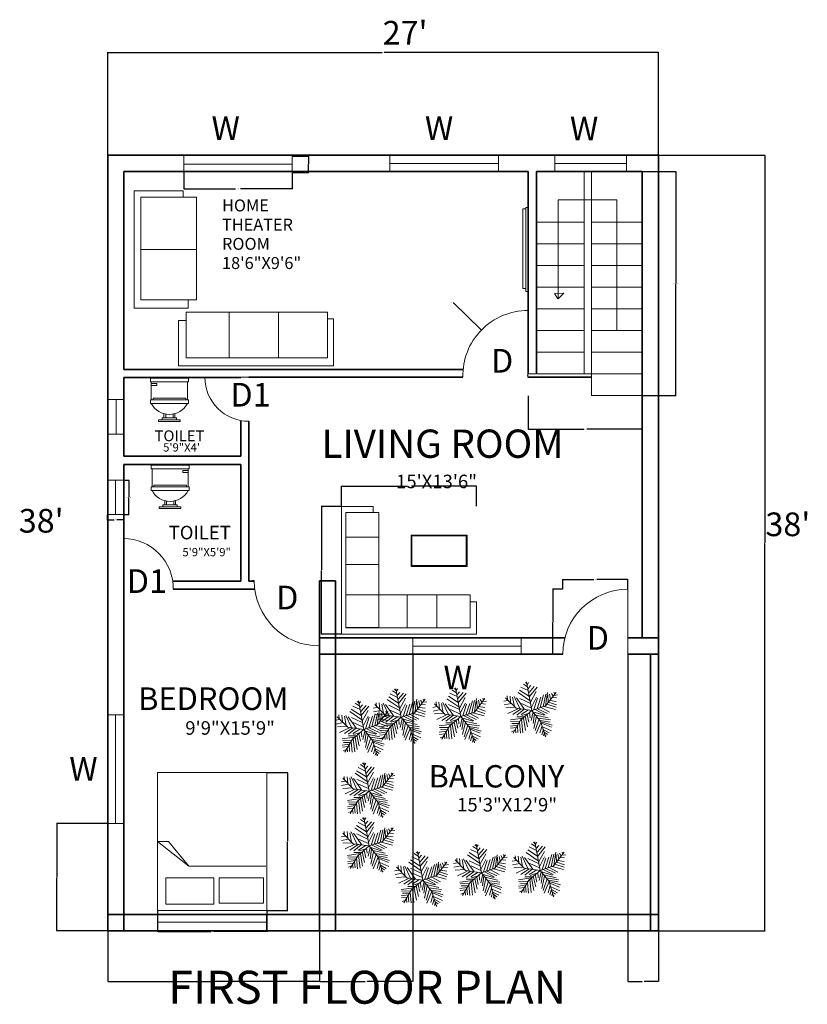
# Model space of a CAD drawing. Units: inches. Extents: x -26 to 788, y -42 to 505.
# Tile 9 of 9: x 353 to 788, y -40 to 505. Entities that reach past the tile are written whole.
import ezdxf

# ---------------------------------------------------------------- set-up
doc = ezdxf.new("R2010")
doc.units = ezdxf.units.IN
doc.header["$MEASUREMENT"] = 0
for name, color, linetype, lineweight in [('A-ANNO-DIMS', 2, 'Continuous', 18), ('A-ANNO-IDEN', 3, 'Continuous', 18), ('A-ANNO-TEXT', 7, 'Continuous', 25), ('A-AREA-IDEN', 7, 'Continuous', 18), ('A-DOOR', 3, 'Continuous', 18), ('A-EQPM', 8, 'Continuous', 18), ('A-FLOR-FIXT', 9, 'Continuous', 18), ('A-FLOR-STRS', 7, 'Continuous', 18), ('A-FURN', 8, 'Continuous', 18), ('A-GLAZ', 4, 'Continuous', 18), ('A-WALL', 7, 'Continuous', 35), ('L-PLNT', 94, 'Continuous', 13)]:
    doc.layers.add(name, color=color, linetype=linetype, lineweight=lineweight)
doc.styles.get("Standard").update_dxf_attribs({"font": 'arial.ttf'})
doc.dimstyles.get("Standard").update_dxf_attribs({"dimtxt": 0.18, "dimasz": 0.18, "dimexe": 0.18, "dimexo": 0.0625, "dimgap": 0.09, "dimtad": 0, "dimtih": 1, "dimtoh": 1, "dimdec": 4, "dimzin": 0, "dimdsep": 46, "dimtxsty": 'Standard', "dimcen": 0.09, "dimadec": 0, "dimazin": 0, "dimtfac": 1, "dimtdec": 4, "dimtofl": 0, "dimtmove": 0, "dimatfit": 3, "dimfxl": 1, "dimtolj": 1, "dimtzin": 0, "dimarcsym": 0})

# ---------------------------------------------------------------- blocks, each defined once
blk = doc.blocks.new('*U2')
for p, q in [((-10, 22), (-10, 12)), ((10, 12), (10, 22)), ((-10, 21), (-7, 21)), ((-7, 20), (-10, 20)), ((-7, 21), (-7, 20)), ((10.5, 12), (-10.5, 12)), ((-10.5, 10), (-10.5, 12)), ((9, 13), (-9, 13)), ((-9, 13), (-9, 12)), ((9, 12), (9, 13)), ((10.5, 12), (10.5, 10)), ((10.5, 10), (-10.5, 10)), ((4, 2), (-4, 2)), ((-4, 2), (-4, 1)), ((-3, 4.4065), (-3, 2)), ((-2, 2), (-2, 4.1658)), ((2, 4.1658), (2, 2)), ((3, 2), (3, 4.4065)), ((4, 1), (4, 2))]:
    blk.add_line(p, q)
for points in [[(10.5, 22), (10.5, 24), (-10.5, 24), (-10.5, 22)], [(6, 0), (6, 1), (-6, 1), (-6, 0)]]:
    blk.add_lwpolyline(points, close=True)
blk.add_arc((0, 15.3333), 11.3333, 208.0725, 331.9275)
blk = doc.blocks.new('*U3')
for p, q in [((-10, 12), (-10, 22)), ((10, 22), (10, 12)), ((10, 21), (7, 21)), ((7, 21), (7, 20)), ((7, 20), (10, 20)), ((-10.5, 12), (10.5, 12)), ((-10.5, 12), (-10.5, 10)), ((-9, 13), (9, 13)), ((-9, 12), (-9, 13)), ((9, 13), (9, 12)), ((10.5, 10), (10.5, 12)), ((-10.5, 10), (10.5, 10)), ((-4, 2), (4, 2)), ((-4, 1), (-4, 2)), ((-3, 2), (-3, 4.4065)), ((-2, 4.1658), (-2, 2)), ((2, 2), (2, 4.1658)), ((3, 4.4065), (3, 2)), ((4, 2), (4, 1))]:
    blk.add_line(p, q)
for points in [[(-10.5, 22), (-10.5, 24), (10.5, 24), (10.5, 22)], [(-6, 0), (-6, 1), (6, 1), (6, 0)]]:
    blk.add_lwpolyline(points, close=True)
blk.add_arc((0, 15.3333), 11.3333, 208.0725, 331.9275)
blk = doc.blocks.new('*D5')
at = {"layer": 'A-ANNO-DIMS', "color": 0, "lineweight": -2, "transparency": 16777216}
for p, q in [((401.21, 429.6), (401.21, 486.57)), ((401.39, 486.39), (552.86, 486.39)), ((705.53, 486.39), (554.07, 486.39)), ((705.71, 429.6), (705.71, 486.57))]:
    blk.add_line(p, q, dxfattribs=at)
at = {"layer": 'A-ANNO-DIMS', "color": 0, "transparency": 16777216}
for points in [[(401.39, 486.42), (401.39, 486.36), (401.21, 486.39)], [(705.53, 486.42), (705.53, 486.36), (705.71, 486.39)]]:
    blk.add_solid(points, dxfattribs=at)
at = {"layer": 'Defpoints', "color": 0, "transparency": 16777216}
for p in [(705.71, 486.39), (401.21, 429.53), (705.71, 429.53)]:
    blk.add_point(p, dxfattribs=at)
at = {"layer": 'A-ANNO-DIMS', "color": 0, "transparency": 16777216, "insert": (553.46, 486.39), "char_height": 0.18, "attachment_point": 5}
blk.add_mtext('\\A1;304.5000', dxfattribs=at)
blk = doc.blocks.new('*D6')
at = {"layer": 'A-ANNO-DIMS', "color": 0, "lineweight": -2, "transparency": 16777216}
for p, q in [((705.78, 429.53), (764.6, 429.53)), ((764.42, 429.35), (764.42, 215.21)), ((764.42, 0.71), (764.42, 214.85)), ((705.78, 0.53), (764.6, 0.53))]:
    blk.add_line(p, q, dxfattribs=at)
at = {"layer": 'A-ANNO-DIMS', "color": 0, "transparency": 16777216}
for points in [[(764.39, 429.35), (764.45, 429.35), (764.42, 429.53)], [(764.39, 0.71), (764.45, 0.71), (764.42, 0.53)]]:
    blk.add_solid(points, dxfattribs=at)
at = {"layer": 'Defpoints', "color": 0, "transparency": 16777216}
for p in [(705.71, 429.53), (705.71, 0.53), (764.42, 0.53)]:
    blk.add_point(p, dxfattribs=at)
at = {"layer": 'A-ANNO-DIMS', "color": 0, "transparency": 16777216, "insert": (764.42, 215.03), "char_height": 0.18, "attachment_point": 5}
blk.add_mtext('\\A1;429.0000', dxfattribs=at)
blk = doc.blocks.new('*U11')
for p, q in [((-129.8956, 713.6638), (-626.7704, 1032.1544)), ((-185.1152, 1008.5578), (-553.1612, 1185.4942)), ((-221.9198, 1197.3052), (-433.5526, 1338.8594)), ((-258.7244, 1362.456), (-332.3336, 1421.4348)), ((0, 0), (-266.7, 1447.8)), ((-231.1146, 1315.2628), (-166.7002, 1421.4348)), ((-194.31, 1102.9442), (-65.4812, 1256.284)), ((-148.3106, 914.1968), (118.5418, 1220.9018)), ((-129.8956, 701.8528), (265.7602, 1185.4942)), ((-1206.4492, 501.3198), (-1418.082, 465.9376)), ((-800.1, 114.3), (-1333.5, 647.7)), ((-1234.059, 536.7274), (-1252.4486, 737.2604)), ((-1105.2302, 725.4494), (-1077.6458, 395.1732)), ((-976.4268, 666.4706), (-884.4026, 194.6402)), ((-902.8176, 713.6638), (-617.5756, 100.2538)), ((-369.1382, 53.086), (-783.1836, 642.874)), ((-93.091, 489.5342), (-700.3796, 902.3858)), ((-617.5756, 607.4918), (-74.7014, 347.98)), ((-74.7014, 418.7444), (219.7608, 961.39)), ((-28.6766, 171.0436), (228.9556, 678.2816)), ((100.1268, 41.275), (284.1498, 619.2774)), ((256.5654, 88.4682), (449.7832, 666.4706)), ((412.9786, 147.447), (587.8068, 796.2392)), ((560.197, 182.8292), (698.2206, 819.8358)), ((685.8, 228.6), (1219.2, 914.4)), ((689.0258, 230.0224), (790.2448, 914.1968)), ((808.6344, 784.4282), (827.0494, 418.7444)), ((891.4384, 831.6214), (946.658, 572.1096)), ((919.0482, 501.3198), (1222.6798, 454.152)), ((983.4626, 867.0036), (1066.2666, 725.4494)), ((1029.462, 654.685), (1241.0948, 631.0884)), ((1112.2914, 760.8316), (1296.3144, 784.4282)), ((1121.4862, 925.9824), (1149.0706, 831.6214)), ((-1031.621, 347.98), (-1399.667, 277.1902)), ((-847.598, 159.2326), (-1326.0578, 135.636)), ((-718.7946, 88.4682), (-1215.644, -147.447)), ((-543.9664, 76.6572), (-967.2066, -206.4512)), ((0, 0), (-800.1, 114.3)), ((-405.9428, 53.086), (-764.794, -241.8334)), ((0, 0), (-571.5, -495.3)), ((-166.7002, 29.4894), (-543.9664, -206.4512)), ((-525.5514, 347.98), (-28.6766, 123.8504)), ((0, 0), (685.8, 228.6)), ((0, 0), (457.2, -571.5)), ((164.5412, 41.275), (661.416, -218.2368)), ((284.1498, 88.4682), (781.0246, -147.447)), ((458.978, 147.447), (891.4384, -88.4682)), ((615.4166, 194.6402), (1185.8752, 41.275)), ((753.4148, 312.5978), (1222.6798, 159.2326)), ((845.439, 418.7444), (1241.0948, 277.1902)), ((-442.7474, -383.3876), (-1086.8406, -477.7486)), ((-571.5, -495.3), (-952.5, -1143)), ((-387.5278, -324.4088), (-764.794, -324.4088)), ((-525.5514, -465.963), (-451.9422, -1126.5408)), ((-166.7002, -147.447), (-507.1618, -253.619)), ((-433.5526, -383.3876), (-323.1134, -1020.3688)), ((-341.5284, -289.0012), (-221.9198, -831.6214)), ((-240.3094, -218.2368), (-157.5054, -595.7062)), ((-120.7008, -88.4682), (-93.091, -371.5766)), ((63.3222, -76.6826), (-37.8714, -513.1308)), ((44.9326, -64.897), (615.4166, -241.8334)), ((127.7366, -159.258), (54.1274, -654.685)), ((228.9556, -289.0012), (90.932, -914.1968)), ((357.759, -430.5554), (164.5412, -1020.3688)), ((192.151, -230.0224), (817.8292, -371.5766)), ((311.7596, -383.3876), (937.4378, -477.7486)), ((-718.7946, -737.2604), (-1086.8406, -796.2392)), ((-617.5756, -548.5384), (-1077.6458, -560.324)), ((-783.1836, -867.029), (-1077.6458, -902.4112)), ((-681.9646, -666.496), (-1022.4262, -654.685)), ((-829.2084, -937.7934), (-810.7934, -1126.5408)), ((-737.1842, -784.4536), (-709.5744, -1114.7298)), ((-635.9652, -607.5172), (-580.771, -1150.1374)), ((458.978, -572.1096), (210.5406, -1161.923)), ((514.1976, -772.6426), (403.7838, -1138.3264)), ((412.9786, -501.3452), (919.0482, -583.9206)), ((457.2, -571.5), (685.8, -1333.5)), ((468.1982, -572.1096), (1029.462, -737.2604)), ((486.5878, -642.8994), (983.4626, -843.4324)), ((578.612, -961.39), (495.7826, -1232.7128)), ((541.8074, -831.6214), (992.6574, -1032.1544)), ((578.612, -973.1756), (873.0488, -1138.3264)), ((-875.2078, -1008.5832), (-1040.8412, -1079.3476)), ((624.6114, -1161.923), (587.8068, -1291.6916)), ((624.6114, -1102.9442), (781.0246, -1209.1162)), ((679.8056, -1268.095), (716.6102, -1291.6916))]:
    blk.add_line(p, q)
blk = doc.blocks.new('WIN-SLIDER-60')
for p, q in [((0, 9), (0, 0)), ((60, 9), (60, 0)), ((0, 4.5), (60, 4.5)), ((60, 4.5), (50.65, 4.5))]:
    blk.add_line(p, q)
blk = doc.blocks.new('WIN-STAIR')
for p, q in [((0, 9), (0, 0)), ((39.57, 9), (39.57, 0)), ((0, 4.5), (39.58, 4.5))]:
    blk.add_line(p, q)
blk = doc.blocks.new('VENT-BATH')
for p, q in [((9, 19.08), (0, 19.08)), ((4.5, 19.08), (4.5, 0)), ((9, 0), (0, 0))]:
    blk.add_line(p, q)
blk = doc.blocks.new('WIN-FIXED-60')
for p, q in [((0, 9), (0, 0)), ((60, 9), (60, 0)), ((0, 4.5), (60, 4.5))]:
    blk.add_line(p, q)
blk = doc.blocks.new('DOOR-BEDROOM-36')
blk.add_line((36, 0), (36, 36))
blk.add_arc((36, 36), 36, 180, 270)
blk = doc.blocks.new('DOOR-ENTRY-36')
blk.add_line((36, 0), (36, 36))
blk.add_arc((36, 0), 36, 90, 179.8595)
blk = doc.blocks.new('DOOR-BATH-A')
blk.add_line((0, 27.99), (0, 0.5))
blk.add_arc((0, 0.5), 27.49, 358.9575, 90)
blk = doc.blocks.new('DOOR-BATH-B')
blk.add_line((24.41, 24.41), (0, 24.41))
blk.add_arc((24.41, 24.41), 24.41, 180, 270)
blk = doc.blocks.new('SOFA-SECTIONAL')
for p, q in [((0, 17.98), (0, 70.62)), ((0, 70.62), (17.39, 70.62)), ((17.39, 70.62), (17.39, 67.34)), ((2.33, 53.68), (20.61, 53.68)), ((2.33, 38.52), (20.61, 38.52)), ((36.15, 21.72), (36.15, 3.64)), ((52.61, 21.72), (52.61, 3.64))]:
    blk.add_line(p, q)
for points in [[(2.33, 3.73), (20.67, 3.73), (20.67, 67.34), (2.33, 67.34)], [(2.32, 21.71), (71.08, 21.71), (71.08, 3.56), (2.32, 3.56)]]:
    blk.add_lwpolyline(points, close=True)
blk.add_lwpolyline([(71.08, 17.8), (74.64, 17.8), (74.64, 0), (0, 0), (0, 17.98)])
blk = doc.blocks.new('BED-DOUBLE')
for p, q in [((17.3, 24.61), (0, 38.23)), ((0, 38.23), (6.1, 38.23)), ((6.1, 38.23), (17.3, 24.61)), ((59.83, 24.61), (17.3, 24.61))]:
    blk.add_line(p, q)
for points in [[(0, 0), (60.34, 0), (60.34, 76.46), (0, 76.46)], [(4.51, 18.22), (31.05, 18.22), (31.05, 3.53), (4.51, 3.53)], [(33.93, 18.22), (58.56, 18.22), (58.56, 4.17), (33.93, 4.17)]]:
    blk.add_lwpolyline(points, close=True)
blk = doc.blocks.new('TABLE-COFFEE')
for points in [[(0, 17.36), (30.93, 17.36), (30.93, 0), (0, 0)], [(0.5, 16.86), (30.43, 16.86), (30.43, 0.5), (0.5, 0.5)]]:
    blk.add_lwpolyline(points, close=True)
blk = doc.blocks.new('STAIR-RETURN')
for p, q in [((30.9, 12), (30.9, 123.91)), ((34.9, 0), (34.9, 123.91)), ((4.5, 96), (30.9, 96)), ((34.9, 96), (63, 96)), ((4.5, 84), (30.9, 84)), ((34.9, 84), (63, 84)), ((4.5, 72), (30.9, 72)), ((34.9, 72), (63, 72)), ((4.5, 60), (30.9, 60)), ((34.9, 60), (63, 60)), ((4.5, 48), (30.9, 48)), ((34.9, 48), (63, 48)), ((4.5, 36), (30.9, 36)), ((34.9, 36), (63, 36)), ((4.5, 24), (30.9, 24)), ((34.9, 24), (63, 24)), ((0, 12), (63, 12)), ((34.9, 0), (63, 0))]:
    blk.add_line(p, q)
blk.add_lwpolyline([(48.95, 36), (48.95, 108.21), (16.43, 108.21), (16.43, 53.45), (19.67, 56.58), (14.49, 56.53), (16.4, 53.46)])
blk = doc.blocks.new('*D27')
at = {"layer": 'A-ANNO-DIMS', "color": 0, "lineweight": -2, "transparency": 16777216}
for p, q in [((443.22, 419.98), (443.22, 410.87)), ((503.22, 419.98), (503.22, 410.87)), ((443.4, 411.05), (471.89, 411.05)), ((503.04, 411.05), (474.55, 411.05))]:
    blk.add_line(p, q, dxfattribs=at)
at = {"layer": 'A-ANNO-DIMS', "color": 0, "transparency": 16777216}
for points in [[(443.4, 411.08), (443.4, 411.02), (443.22, 411.05)], [(503.04, 411.08), (503.04, 411.02), (503.22, 411.05)]]:
    blk.add_solid(points, dxfattribs=at)
at = {"layer": 'Defpoints', "color": 0, "transparency": 16777216}
for p in [(443.22, 420.05), (503.22, 420.05), (503.22, 411.05)]:
    blk.add_point(p, dxfattribs=at)
at = {"layer": 'A-ANNO-DIMS', "color": 0, "transparency": 16777216, "insert": (473.22, 411.05), "char_height": 0.18, "attachment_point": 5}
blk.add_mtext('\\A1;SLIDER 60.0000 TYP.', dxfattribs=at)
blk = doc.blocks.new('*D28')
at = {"layer": 'A-ANNO-DIMS', "color": 0, "lineweight": -2, "transparency": 16777216}
for p, q in [((503.28, 429.05), (512.4, 429.05)), ((512.22, 428.87), (512.22, 424.73)), ((503.28, 420.05), (512.4, 420.05)), ((512.22, 420.23), (512.22, 424.37))]:
    blk.add_line(p, q, dxfattribs=at)
at = {"layer": 'A-ANNO-DIMS', "color": 0, "transparency": 16777216}
for points in [[(512.19, 428.87), (512.25, 428.87), (512.22, 429.05)], [(512.19, 420.23), (512.25, 420.23), (512.22, 420.05)]]:
    blk.add_solid(points, dxfattribs=at)
at = {"layer": 'Defpoints', "color": 0, "transparency": 16777216}
for p in [(503.22, 429.05), (512.22, 429.05), (503.22, 420.05)]:
    blk.add_point(p, dxfattribs=at)
at = {"layer": 'A-ANNO-DIMS', "color": 0, "transparency": 16777216, "insert": (512.22, 424.55), "char_height": 0.18, "attachment_point": 5}
blk.add_mtext('\\A1;9.0000 TYP.', dxfattribs=at)
blk = doc.blocks.new('*D29')
at = {"layer": 'A-ANNO-DIMS', "color": 0, "lineweight": -2, "transparency": 16777216}
for p, q in [((410.05, 249.88), (413.03, 249.88)), ((412.85, 249.7), (412.85, 240.52)), ((412.85, 230.98), (412.85, 240.15)), ((410.05, 230.8), (413.03, 230.8))]:
    blk.add_line(p, q, dxfattribs=at)
at = {"layer": 'A-ANNO-DIMS', "color": 0, "transparency": 16777216}
for points in [[(412.82, 249.7), (412.88, 249.7), (412.85, 249.88)], [(412.82, 230.98), (412.88, 230.98), (412.85, 230.8)]]:
    blk.add_solid(points, dxfattribs=at)
at = {"layer": 'Defpoints', "color": 0, "transparency": 16777216}
for p in [(409.99, 249.88), (412.85, 249.88), (409.99, 230.8)]:
    blk.add_point(p, dxfattribs=at)
at = {"layer": 'A-ANNO-DIMS', "color": 0, "transparency": 16777216, "insert": (412.85, 240.34), "char_height": 0.18, "attachment_point": 5}
blk.add_mtext('\\A1;BATH VENT 19.0786 TYP.', dxfattribs=at)
blk = doc.blocks.new('*D30')
at = {"layer": 'A-ANNO-DIMS', "color": 0, "lineweight": -2, "transparency": 16777216}
for p, q in [((400.99, 230.73), (400.99, 227.76)), ((409.99, 230.73), (409.99, 227.76)), ((401.17, 227.94), (404.71, 227.94)), ((409.81, 227.94), (406.26, 227.94))]:
    blk.add_line(p, q, dxfattribs=at)
at = {"layer": 'A-ANNO-DIMS', "color": 0, "transparency": 16777216}
for points in [[(401.17, 227.97), (401.17, 227.91), (400.99, 227.94)], [(409.81, 227.97), (409.81, 227.91), (409.99, 227.94)]]:
    blk.add_solid(points, dxfattribs=at)
at = {"layer": 'Defpoints', "color": 0, "transparency": 16777216}
for p in [(400.99, 230.8), (409.99, 230.8), (409.99, 227.94)]:
    blk.add_point(p, dxfattribs=at)
at = {"layer": 'A-ANNO-DIMS', "color": 0, "transparency": 16777216, "insert": (405.49, 227.94), "char_height": 0.18, "attachment_point": 5}
blk.add_mtext('\\A1;9.0000 TYP.', dxfattribs=at)
blk = doc.blocks.new('*D37')
at = {"layer": 'A-ANNO-DIMS', "color": 0, "lineweight": -2, "transparency": 16777216}
for p, q in [((652.67, 189.44), (647.16, 189.44)), ((647.34, 189.26), (647.34, 171.63)), ((647.34, 153.62), (647.34, 171.26)), ((652.67, 153.44), (647.16, 153.44))]:
    blk.add_line(p, q, dxfattribs=at)
at = {"layer": 'A-ANNO-DIMS', "color": 0, "transparency": 16777216}
for points in [[(647.31, 189.26), (647.37, 189.26), (647.34, 189.44)], [(647.31, 153.62), (647.37, 153.62), (647.34, 153.44)]]:
    blk.add_solid(points, dxfattribs=at)
at = {"layer": 'Defpoints', "color": 0, "transparency": 16777216}
for p in [(647.34, 189.44), (652.74, 189.44), (652.74, 153.44)]:
    blk.add_point(p, dxfattribs=at)
at = {"layer": 'A-ANNO-DIMS', "color": 0, "transparency": 16777216, "insert": (647.34, 171.44), "char_height": 0.18, "attachment_point": 5}
blk.add_mtext('\\A1;ENTRY DOOR 36.0000 TYP.', dxfattribs=at)
blk = doc.blocks.new('*D38')
at = {"layer": 'A-ANNO-DIMS', "color": 0, "lineweight": -2, "transparency": 16777216}
for p, q in [((652.74, 189.51), (652.74, 195.02)), ((652.92, 194.84), (669.89, 194.84)), ((688.56, 194.84), (671.58, 194.84)), ((688.74, 189.51), (688.74, 195.02))]:
    blk.add_line(p, q, dxfattribs=at)
at = {"layer": 'A-ANNO-DIMS', "color": 0, "transparency": 16777216}
for points in [[(652.92, 194.87), (652.92, 194.81), (652.74, 194.84)], [(688.56, 194.87), (688.56, 194.81), (688.74, 194.84)]]:
    blk.add_solid(points, dxfattribs=at)
at = {"layer": 'Defpoints', "color": 0, "transparency": 16777216}
for p in [(688.74, 194.84), (652.74, 189.44), (688.74, 189.44)]:
    blk.add_point(p, dxfattribs=at)
at = {"layer": 'A-ANNO-DIMS', "color": 0, "transparency": 16777216, "insert": (670.74, 194.84), "char_height": 0.18, "attachment_point": 5}
blk.add_mtext('\\A1;35.9999 TYP.', dxfattribs=at)
blk = doc.blocks.new('*D43')
at = {"layer": 'A-ANNO-DIMS', "color": 0, "lineweight": -2, "transparency": 16777216}
for p, q in [((530.5, 235.35), (530.5, 246.66)), ((530.68, 246.48), (566.61, 246.48)), ((604.97, 246.48), (569.05, 246.48)), ((605.15, 235.35), (605.15, 246.66))]:
    blk.add_line(p, q, dxfattribs=at)
at = {"layer": 'A-ANNO-DIMS', "color": 0, "transparency": 16777216}
for points in [[(530.68, 246.51), (530.68, 246.45), (530.5, 246.48)], [(604.97, 246.51), (604.97, 246.45), (605.15, 246.48)]]:
    blk.add_solid(points, dxfattribs=at)
at = {"layer": 'Defpoints', "color": 0, "transparency": 16777216}
for p in [(605.15, 246.48), (530.5, 235.29), (605.15, 235.29)]:
    blk.add_point(p, dxfattribs=at)
at = {"layer": 'A-ANNO-DIMS', "color": 0, "transparency": 16777216, "insert": (567.83, 246.48), "char_height": 0.18, "attachment_point": 5}
blk.add_mtext('\\A1;SOFA 74.6433 TYP.', dxfattribs=at)
blk = doc.blocks.new('*D44')
at = {"layer": 'A-ANNO-DIMS', "color": 0, "lineweight": -2, "transparency": 16777216}
for p, q in [((530.44, 235.29), (519.13, 235.29)), ((519.31, 235.11), (519.31, 200.16)), ((519.31, 164.84), (519.31, 199.79)), ((530.44, 164.66), (519.13, 164.66))]:
    blk.add_line(p, q, dxfattribs=at)
at = {"layer": 'A-ANNO-DIMS', "color": 0, "transparency": 16777216}
for points in [[(519.28, 235.11), (519.34, 235.11), (519.31, 235.29)], [(519.28, 164.84), (519.34, 164.84), (519.31, 164.66)]]:
    blk.add_solid(points, dxfattribs=at)
at = {"layer": 'Defpoints', "color": 0, "transparency": 16777216}
for p in [(519.31, 235.29), (530.5, 235.29), (530.5, 164.66)]:
    blk.add_point(p, dxfattribs=at)
at = {"layer": 'A-ANNO-DIMS', "color": 0, "transparency": 16777216, "insert": (519.31, 199.98), "char_height": 0.18, "attachment_point": 5}
blk.add_mtext('\\A1;70.6222 TYP.', dxfattribs=at)
blk = doc.blocks.new('*D45')
at = {"layer": 'A-ANNO-DIMS', "color": 0, "lineweight": -2, "transparency": 16777216}
for p, q in [((489.21, 88.14), (500.8, 88.14)), ((500.62, 87.96), (500.62, 50.09)), ((500.62, 11.86), (500.62, 49.73)), ((489.21, 11.68), (500.8, 11.68))]:
    blk.add_line(p, q, dxfattribs=at)
at = {"layer": 'A-ANNO-DIMS', "color": 0, "transparency": 16777216}
for points in [[(500.59, 87.96), (500.65, 87.96), (500.62, 88.14)], [(500.59, 11.86), (500.65, 11.86), (500.62, 11.68)]]:
    blk.add_solid(points, dxfattribs=at)
at = {"layer": 'Defpoints', "color": 0, "transparency": 16777216}
for p in [(489.15, 88.14), (500.62, 88.14), (489.15, 11.68)]:
    blk.add_point(p, dxfattribs=at)
at = {"layer": 'A-ANNO-DIMS', "color": 0, "transparency": 16777216, "insert": (500.62, 49.91), "char_height": 0.18, "attachment_point": 5}
blk.add_mtext('\\A1;DOUBLE BED 76.4634 TYP.', dxfattribs=at)
blk = doc.blocks.new('*D46')
at = {"layer": 'A-ANNO-DIMS', "color": 0, "lineweight": -2, "transparency": 16777216}
for p, q in [((428.81, 11.62), (428.81, 0.03)), ((489.15, 11.62), (489.15, 0.03)), ((428.99, 0.21), (458.14, 0.21)), ((488.97, 0.21), (459.82, 0.21))]:
    blk.add_line(p, q, dxfattribs=at)
at = {"layer": 'A-ANNO-DIMS', "color": 0, "transparency": 16777216}
for points in [[(428.99, 0.24), (428.99, 0.18), (428.81, 0.21)], [(488.97, 0.24), (488.97, 0.18), (489.15, 0.21)]]:
    blk.add_solid(points, dxfattribs=at)
at = {"layer": 'Defpoints', "color": 0, "transparency": 16777216}
for p in [(428.81, 11.68), (489.15, 11.68), (489.15, 0.21)]:
    blk.add_point(p, dxfattribs=at)
at = {"layer": 'A-ANNO-DIMS', "color": 0, "transparency": 16777216, "insert": (458.98, 0.21), "char_height": 0.18, "attachment_point": 5}
blk.add_mtext('\\A1;60.3394 TYP.', dxfattribs=at)
blk = doc.blocks.new('*D49')
at = {"layer": 'A-ANNO-DIMS', "color": 0, "lineweight": -2, "transparency": 16777216}
for p, q in [((696.78, 420.53), (715.48, 420.53)), ((715.3, 420.35), (715.3, 358.76)), ((715.3, 296.8), (715.3, 358.39)), ((696.78, 296.62), (715.48, 296.62))]:
    blk.add_line(p, q, dxfattribs=at)
at = {"layer": 'A-ANNO-DIMS', "color": 0, "transparency": 16777216}
for points in [[(715.27, 420.35), (715.33, 420.35), (715.3, 420.53)], [(715.27, 296.8), (715.33, 296.8), (715.3, 296.62)]]:
    blk.add_solid(points, dxfattribs=at)
at = {"layer": 'Defpoints', "color": 0, "transparency": 16777216}
for p in [(696.71, 420.53), (715.3, 420.53), (696.71, 296.62)]:
    blk.add_point(p, dxfattribs=at)
at = {"layer": 'A-ANNO-DIMS', "color": 0, "transparency": 16777216, "insert": (715.3, 358.58), "char_height": 0.18, "attachment_point": 5}
blk.add_mtext('\\A1;RETURN STAIR 123.9147 TYP.', dxfattribs=at)
blk = doc.blocks.new('*D50')
at = {"layer": 'A-ANNO-DIMS', "color": 0, "lineweight": -2, "transparency": 16777216}
for p, q in [((633.71, 296.56), (633.71, 277.85)), ((696.71, 296.56), (696.71, 277.85)), ((633.89, 278.03), (664.37, 278.03)), ((696.53, 278.03), (666.06, 278.03))]:
    blk.add_line(p, q, dxfattribs=at)
at = {"layer": 'A-ANNO-DIMS', "color": 0, "transparency": 16777216}
for points in [[(633.89, 278.06), (633.89, 278), (633.71, 278.03)], [(696.53, 278.06), (696.53, 278), (696.71, 278.03)]]:
    blk.add_solid(points, dxfattribs=at)
at = {"layer": 'Defpoints', "color": 0, "transparency": 16777216}
for p in [(633.71, 296.62), (696.71, 296.62), (696.71, 278.03)]:
    blk.add_point(p, dxfattribs=at)
at = {"layer": 'A-ANNO-DIMS', "color": 0, "transparency": 16777216, "insert": (665.21, 278.03), "char_height": 0.18, "attachment_point": 5}
blk.add_mtext('\\A1;63.0000 TYP.', dxfattribs=at)
blk = doc.blocks.new('*D51')
at = {"layer": 'A-ANNO-DIMS', "color": 0, "lineweight": -2, "transparency": 16777216}
for p, q in [((401.21, 0.47), (401.21, -27.6)), ((518.21, 0.47), (518.21, -27.6)), ((401.39, -27.42), (459.12, -27.42)), ((518.03, -27.42), (460.31, -27.42))]:
    blk.add_line(p, q, dxfattribs=at)
at = {"layer": 'A-ANNO-DIMS', "color": 0, "transparency": 16777216}
for points in [[(401.39, -27.39), (401.39, -27.45), (401.21, -27.42)], [(518.03, -27.39), (518.03, -27.45), (518.21, -27.42)]]:
    blk.add_solid(points, dxfattribs=at)
at = {"layer": 'Defpoints', "color": 0, "transparency": 16777216}
for p in [(401.21, 0.53), (518.21, 0.53), (518.21, -27.42)]:
    blk.add_point(p, dxfattribs=at)
at = {"layer": 'A-ANNO-DIMS', "color": 0, "transparency": 16777216, "insert": (459.71, -27.42), "char_height": 0.18, "attachment_point": 5}
blk.add_mtext('\\A1;117.0000', dxfattribs=at)
blk = doc.blocks.new('*D57')
at = {"layer": 'A-ANNO-DIMS', "color": 0, "lineweight": -2, "transparency": 16777216}
for p, q in [((401.02, 59.95), (372.86, 59.95)), ((373.04, 59.77), (373.04, 30.42)), ((373.04, 0.71), (373.04, 30.06)), ((401.15, 0.53), (372.86, 0.53))]:
    blk.add_line(p, q, dxfattribs=at)
at = {"layer": 'A-ANNO-DIMS', "color": 0, "transparency": 16777216}
for points in [[(373.01, 59.77), (373.07, 59.77), (373.04, 59.95)], [(373.01, 0.71), (373.07, 0.71), (373.04, 0.53)]]:
    blk.add_solid(points, dxfattribs=at)
at = {"layer": 'Defpoints', "color": 0, "transparency": 16777216}
for p in [(373.04, 59.95), (401.09, 59.95), (401.21, 0.53)]:
    blk.add_point(p, dxfattribs=at)
at = {"layer": 'A-ANNO-DIMS', "color": 0, "transparency": 16777216, "insert": (373.04, 30.24), "char_height": 0.18, "attachment_point": 5}
blk.add_mtext('\\A1;59.4133', dxfattribs=at)
blk = doc.blocks.new('*D58')
at = {"layer": 'A-ANNO-DIMS', "color": 0, "lineweight": -2, "transparency": 16777216}
for p, q in [((688.74, 153.38), (688.74, -27.6)), ((705.71, 153.47), (705.71, -27.6)), ((688.92, -27.42), (696.7, -27.42)), ((705.53, -27.42), (697.75, -27.42))]:
    blk.add_line(p, q, dxfattribs=at)
at = {"layer": 'A-ANNO-DIMS', "color": 0, "transparency": 16777216}
for points in [[(688.92, -27.39), (688.92, -27.45), (688.74, -27.42)], [(705.53, -27.39), (705.53, -27.45), (705.71, -27.42)]]:
    blk.add_solid(points, dxfattribs=at)
at = {"layer": 'Defpoints', "color": 0, "transparency": 16777216}
for p in [(688.74, 153.44), (705.71, 153.53), (705.71, -27.42)]:
    blk.add_point(p, dxfattribs=at)
at = {"layer": 'A-ANNO-DIMS', "color": 0, "transparency": 16777216, "insert": (697.22, -27.42), "char_height": 0.18, "attachment_point": 5}
blk.add_mtext('\\A1;16.9774', dxfattribs=at)
blk = doc.blocks.new('*D59')
at = {"layer": 'A-ANNO-DIMS', "color": 0, "lineweight": -2, "transparency": 16777216}
for p, q in [((518.21, 153.47), (518.21, -27.6)), ((569.83, 153.43), (569.83, -27.6)), ((518.39, -27.42), (543.49, -27.42)), ((569.65, -27.42), (544.56, -27.42))]:
    blk.add_line(p, q, dxfattribs=at)
at = {"layer": 'A-ANNO-DIMS', "color": 0, "transparency": 16777216}
for points in [[(518.39, -27.39), (518.39, -27.45), (518.21, -27.42)], [(569.65, -27.39), (569.65, -27.45), (569.83, -27.42)]]:
    blk.add_solid(points, dxfattribs=at)
at = {"layer": 'Defpoints', "color": 0, "transparency": 16777216}
for p in [(518.21, 153.53), (569.83, 153.5), (569.83, -27.42)]:
    blk.add_point(p, dxfattribs=at)
at = {"layer": 'A-ANNO-DIMS', "color": 0, "transparency": 16777216, "insert": (544.02, -27.42), "char_height": 0.18, "attachment_point": 5}
blk.add_mtext('\\A1;51.6214', dxfattribs=at)
blk = doc.blocks.new('*D68')
at = {"layer": 'A-ANNO-DIMS', "color": 0, "lineweight": -2, "transparency": 16777216}
for p, q in [((592.1, 347.91), (592.28, 347.91)), ((592.28, 347.91), (607.62, 332.95)), ((633.43, 307.69), (633.61, 307.69)), ((633.52, 307.6), (633.52, 307.78))]:
    blk.add_line(p, q, dxfattribs=at)
at = {"layer": 'A-ANNO-DIMS', "color": 0, "transparency": 16777216}
blk.add_solid([(607.64, 332.97), (607.6, 332.93), (607.74, 332.83)], dxfattribs=at)
at = {"layer": 'Defpoints', "color": 0, "transparency": 16777216}
for p in [(607.74, 332.83), (633.52, 307.69)]:
    blk.add_point(p, dxfattribs=at)
at = {"layer": 'A-ANNO-DIMS', "color": 0, "transparency": 16777216, "insert": (591.29, 347.91), "char_height": 0.18, "attachment_point": 5}
blk.add_mtext('\\A1;5X R36.0000', dxfattribs=at)

msp = doc.modelspace()

# ---------------------------------------------------------------- linework, layer by layer
at = {"layer": 'A-DOOR'}
msp.add_line((633.51795, 306.78903), (633.51795, 343.6915), dxfattribs=at)
msp.add_arc((633.51795, 307.6915), 36, 90, 181.4364755, dxfattribs=at)
at = {"layer": 'A-EQPM'}
for points in [[(632.37277, 399.99815), (630.72584, 399.99815), (630.72584, 355.84706), (632.37277, 355.84706)], [(633.65712, 400.65621), (632.34883, 400.65621), (632.34883, 354.25566), (633.65712, 354.25566)]]:
    msp.add_lwpolyline(points, close=True, dxfattribs=at)
at = {"layer": 'A-FURN'}
for p, q in [((419.58403, 377.46533), (450.04128, 377.46533)), ((468.40202, 342.72078), (468.40202, 317.47163)), ((495.61911, 342.72078), (495.61911, 317.47163))]:
    msp.add_line(p, q, dxfattribs=at)
for points in [[(442.91298, 406.59896), (442.91298, 409.83603), (415.91188, 409.83603), (415.91188, 344.87883), (445.72109, 344.87883), (445.72109, 348.54751), (445.72109, 349.62653)], [(444.42503, 338.18888), (440.32088, 338.18888), (440.32088, 313.15555), (526.07636, 313.15555), (526.07636, 339.0521), (522.62022, 339.0521)]]:
    msp.add_lwpolyline(points, dxfattribs=at)
for points in [[(419.58403, 406.38315), (450.25729, 406.38315), (450.25729, 349.62653), (419.58403, 349.62653)], [(444.64104, 342.72078), (522.62022, 342.72078), (522.62022, 317.47163), (444.64104, 317.47163)]]:
    msp.add_lwpolyline(points, close=True, dxfattribs=at)
at = {"layer": 'A-WALL'}
for p, q in [((401.21324, 429.53259), (705.71324, 429.53259)), ((401.21324, 0.53259), (401.21324, 429.53259)), ((705.71324, 306.78903), (705.71324, 429.53259)), ((410.21324, 420.53259), (527.21324, 420.53259)), ((410.21324, 311.03259), (410.21324, 420.53259)), ((527.21324, 420.53259), (633.71324, 420.53259)), ((633.71324, 308.61788), (633.71324, 420.53259)), ((638.21324, 420.53259), (696.71324, 420.53259)), ((638.21324, 308.61788), (638.21324, 420.53259)), ((696.71324, 162.53259), (696.71324, 420.53259)), ((410.21324, 311.03259), (597.67332, 311.03259)), ((633.51795, 311.03259), (633.71324, 311.03259)), ((410.21324, 306.53259), (474.71324, 306.53259)), ((410.21324, 263.03259), (410.21324, 306.53259)), ((479.21324, 306.78903), (597.52926, 306.78903)), ((633.51795, 306.78903), (668.61324, 306.78903)), ((705.71324, 0.53259), (705.71324, 306.78903)), ((474.71324, 263.03259), (474.71324, 282.81802)), ((479.21324, 194.03259), (479.21324, 282.38179)), ((410.21324, 263.03259), (474.71324, 263.03259)), ((410.21324, 258.53259), (474.71324, 258.53259)), ((410.21324, 0.53259), (410.21324, 258.53259)), ((474.71324, 194.03259), (474.71324, 258.53259)), ((437.14055, 194.03259), (474.71324, 194.03259)), ((479.21324, 194.03259), (482.21336, 194.03259)), ((482.21324, 194.12381), (481.25581, 194.12381)), ((518.21324, 0.53259), (518.21324, 194.12381)), ((527.21324, 194.12381), (518.21324, 194.12381)), ((527.21324, 0.53259), (527.21324, 194.12381)), ((409.93933, 190.0328), (410.21324, 190.029)), ((437.4285, 189.53259), (482.50721, 189.53259)), ((518.21324, 162.53259), (653.90189, 162.53259)), ((688.73583, 162.53259), (705.71324, 162.53259)), ((518.21324, 153.53259), (652.73594, 153.53259)), ((688.73583, 153.53259), (705.71324, 153.53259)), ((701.21324, 0.53259), (701.21324, 153.53259)), ((401.21324, 9.53259), (705.71324, 9.53259)), ((401.21324, 0.53259), (705.71324, 0.53259))]:
    msp.add_line(p, q, dxfattribs=at)

# ---------------------------------------------------------------- block references
at = {"layer": 'A-DOOR'}
for name, p in [('DOOR-BATH-B', (454.90028, 282.38182)), ('DOOR-BATH-A', (409.93928, 189.53282)), ('DOOR-BEDROOM-36', (482.21328, 158.12382)), ('DOOR-ENTRY-36', (652.73628, 153.44482))]:
    msp.add_blockref(name, p, dxfattribs=at)
at = {"layer": 'A-FLOR-FIXT'}
for name, p in [('*U2', (435.3124, 282.22509)), ('*U3', (435.70247, 234.0998))]:
    msp.add_blockref(name, p, dxfattribs=at)
at = {"layer": 'A-FLOR-STRS'}
msp.add_blockref('STAIR-RETURN', (633.71328, 296.61782), dxfattribs=at)
at = {"layer": 'A-FURN'}
for name, p in [('SOFA-SECTIONAL', (530.50428, 164.66382)), ('TABLE-COFFEE', (568.89328, 202.11882)), ('BED-DOUBLE', (428.81028, 11.67782))]:
    msp.add_blockref(name, p, dxfattribs=at)
at = {"layer": 'A-GLAZ'}
for name, p in [('WIN-SLIDER-60', (443.21671, 420.047)), ('WIN-SLIDER-60', (557.17398, 420.57901)), ('WIN-STAIR', (648.34128, 420.50082)), ('VENT-BATH', (401.43075, 275.30093)), ('VENT-BATH', (400.98528, 230.79682)), ('WIN-SLIDER-60', (569.83428, 153.49682)), ('WIN-FIXED-60', (428.92628, 0.78682))]:
    msp.add_blockref(name, p, dxfattribs=at)
at = {"layer": 'A-GLAZ', "rotation": 270}
msp.add_blockref('WIN-SLIDER-60', (401.0851, 119.94634), dxfattribs=at)
at = {"layer": 'L-PLNT', "xscale": 0.0109273732196715, "yscale": 0.0109273732196715, "zscale": 0.0109273732196715}
for p in [(635.71227, 122.42221), (563.37018, 118.64451), (596.39892, 119.06221), (542.70916, 111.89985), (545.67713, 77.82816), (545.67713, 47.47039), (640.21284, 33.97805), (575.38835, 28.58112), (607.80058, 32.62882)]:
    msp.add_blockref('*U11', p, dxfattribs=at)

# ---------------------------------------------------------------- texts
at = {"layer": 'A-ANNO-DIMS'}
for s, p in [("27'", (553.20541, 490.77036)), ("38'", (352.05662, 220.79894)), ("38'", (764.76948, 218.84996))]:
    msp.add_text(s, height=13.093175, dxfattribs=at).set_placement(p)
at = {"layer": 'A-ANNO-IDEN'}
for s, height, p in [('W', 13.09317, (458.59921, 438.01998)), ('W', 13.09317, (576.54914, 438.01998)), ('W', 13.09317, (656.70939, 437.76162)), ('D', 13.09317, (613.08535, 309.30061)), ('D1', 13.093175, (469.06806, 290.50797)), ('D1', 13.093175, (411.75786, 187.42721)), ('D', 13.09317, (494.34459, 178.33934)), ('D', 13.09317, (665.98967, 156.02308)), ('W', 13.09317, (586.84635, 134.07146)), ('W', 13.09317, (379.9659, 83.56925))]:
    msp.add_text(s, height=height, dxfattribs=at).set_placement(p)
at = {"layer": 'A-ANNO-TEXT'}
msp.add_text('FIRST FLOOR PLAN', height=18.2344212, dxfattribs=at).set_placement((434.64946, -39.80114))
at = {"layer": 'A-AREA-IDEN'}
for s, height, p in [('HOME ', 6.609405, (464.40538, 398.4827)), ('THEATER', 6.609405, (464.40538, 387.86527)), ('ROOM', 6.609405, (464.40538, 377.24784)), ('18\'6"X9\'6"', 6.609405, (464.40538, 366.63041)), ('LIVING ROOM', 15.6450193, (519.35814, 262.16253)), ('TOILET', 6.011917, (427.10279, 271.3473)), ('5\'9"X4\'', 4.56659, (431.8674, 265.66305)), ('15\'X13\'6"', 7.483862, (560.62618, 245.36904)), ('TOILET', 7.483862, (434.94484, 217.09668)), ('5\'9"X5\'9"', 4.56659, (442.5265, 207.73508)), ('BEDROOM', 12.516013, (418.02874, 122.67373)), ('9\'9"X15\'9"', 7.483862, (444.10044, 108.99643)), ('BALCONY', 12.369099, (578.64092, 79.81466)), ('15\'3"X12\'9"', 7.4838625, (594.38013, 66.53643))]:
    msp.add_text(s, height=height, dxfattribs=at).set_placement(p)

# ---------------------------------------------------------------- dimensions: what is measured, and where the dimension line sits
at = {"layer": 'A-ANNO-DIMS'}
for base, p1, p2, override, picture, middle in [((705.71324, 486.39109), (401.21324, 429.53259), (705.71324, 429.53259), {"dimclrd": 0, "dimclre": 0, "dimclrt": 0}, '*D5', (553.46324, 486.39109)), ((569.83468, -27.41741), (518.21324, 153.53259), (569.83468, 153.49675), {"dimdec": 4, "dimlfac": 1, "dimrnd": 0, "dimzin": 0, "dimdsep": 46, "dimlunit": 2}, '*D59', (544.02396, -27.41741)), ((705.71324, -27.41741), (688.73583, 153.44434), (705.71324, 153.53259), {"dimdec": 4, "dimlfac": 1, "dimrnd": 0, "dimzin": 0, "dimdsep": 46, "dimlunit": 2}, '*D58', (697.22454, -27.41741)), ((518.21324, -27.41741), (401.21324, 0.53259), (518.21324, 0.53259), {"dimdec": 4, "dimlfac": 1, "dimrnd": 0, "dimzin": 0, "dimdsep": 46, "dimlunit": 2}, '*D51', (459.71324, -27.41741))]:
    dim = msp.add_linear_dim(base=base, p1=p1, p2=p2, dimstyle='Standard', override=override, dxfattribs=at)
    dim.commit()
    dim.dimension.update_dxf_attribs({"geometry": picture, "text_midpoint": middle})
for base, p1, p2, text, picture, middle in [((512.21712, 429.04693), (503.21712, 420.04693), (503.21712, 429.04693), '<> TYP.', '*D28', (512.21712, 424.54693)), ((715.30045, 420.53259), (696.71324, 296.61788), (696.71324, 420.53259), 'RETURN STAIR <> TYP.', '*D49', (715.30045, 358.57524)), ((412.84721, 249.87538), (409.98542, 230.7968), (409.98542, 249.87538), 'BATH VENT <> TYP.', '*D29', (412.84721, 240.33609)), ((519.30745, 235.28647), (530.50395, 164.66428), (530.50395, 235.28647), '<> TYP.', '*D44', (519.30745, 199.97538)), ((647.33594, 189.44434), (652.73594, 153.44434), (652.73594, 189.44434), 'ENTRY DOOR <> TYP.', '*D37', (647.33594, 171.44434)), ((500.6189, 88.1412), (489.14939, 11.67777), (489.14939, 88.1412), 'DOUBLE BED <> TYP.', '*D45', (500.6189, 49.90948))]:
    dim = msp.add_linear_dim(base=base, p1=p1, p2=p2, angle=90, text=text, dimstyle='Standard', override={"dimdec": 4, "dimlfac": 1, "dimrnd": 0, "dimzin": 0, "dimdsep": 46, "dimlunit": 2}, dxfattribs=at)
    dim.commit()
    dim.dimension.update_dxf_attribs({"geometry": picture, "text_midpoint": middle})
for base, p1, p2, override, picture, middle in [((764.4242, 0.53259), (705.71324, 429.53259), (705.71324, 0.53259), {"dimclrd": 0, "dimclre": 0, "dimclrt": 0}, '*D6', (764.4242, 215.03259)), ((373.035422, 59.945939), (401.213243, 0.532592), (401.085028, 59.945939), {"dimdec": 4, "dimlfac": 1, "dimrnd": 0, "dimzin": 0, "dimdsep": 46, "dimlunit": 2}, '*D57', (373.035422, 30.239265))]:
    dim = msp.add_linear_dim(base=base, p1=p1, p2=p2, angle=90, dimstyle='Standard', override=override, dxfattribs=at)
    dim.commit()
    dim.dimension.update_dxf_attribs({"geometry": picture, "text_midpoint": middle})
for base, p1, p2, text, picture, middle in [((503.21712, 411.04693), (443.21712, 420.04693), (503.21712, 420.04693), 'SLIDER <> TYP.', '*D27', (473.21712, 411.04693)), ((696.71324, 278.03068), (633.71324, 296.61788), (696.71324, 296.61788), '<> TYP.', '*D50', (665.21324, 278.03068)), ((605.147298, 246.482974), (530.50395, 235.286472), (605.147298, 235.286472), 'SOFA <> TYP.', '*D43', (567.825624, 246.482974)), ((409.98542, 227.93501), (400.98542, 230.7968), (409.98542, 230.7968), '<> TYP.', '*D30', (405.48542, 227.93501)), ((688.73583, 194.84434), (652.73594, 189.44434), (688.73583, 189.44434), '<> TYP.', '*D38', (670.73589, 194.84434)), ((489.14939, 0.20825), (428.80999, 11.67777), (489.14939, 11.67777), '<> TYP.', '*D46', (458.97969, 0.20825))]:
    dim = msp.add_linear_dim(base=base, p1=p1, p2=p2, text=text, dimstyle='Standard', override={"dimdec": 4, "dimlfac": 1, "dimrnd": 0, "dimzin": 0, "dimdsep": 46, "dimlunit": 2}, dxfattribs=at)
    dim.commit()
    dim.dimension.update_dxf_attribs({"geometry": picture, "text_midpoint": middle})
dim = msp.add_radius_dim(center=(633.51795, 307.6915), mpoint=(607.74488, 332.82612), text='5X <>', dimstyle='Standard', override={"dimdec": 4, "dimlfac": 1, "dimrnd": 0, "dimzin": 0, "dimdsep": 46, "dimlunit": 2}, dxfattribs=at)
dim.commit()
dim.dimension.update_dxf_attribs({"geometry": '*D68', "text_midpoint": (591.28828, 347.90689), "dimtype": 164})

doc.saveas('drawing.dxf')
